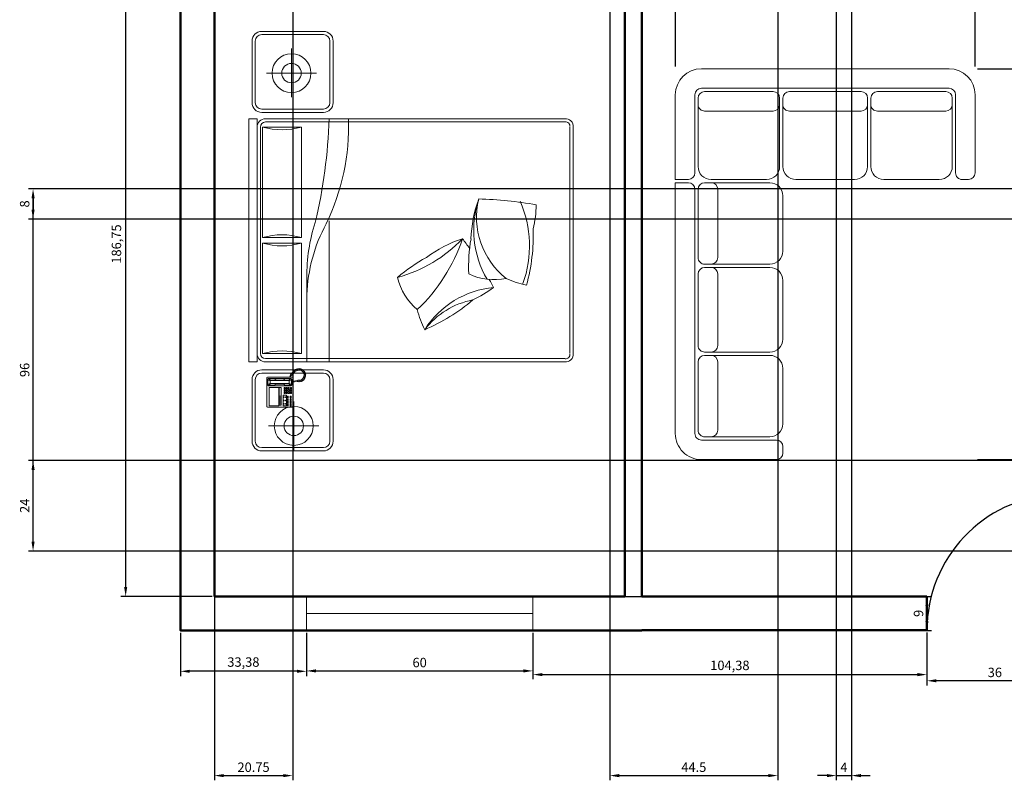
# Model space of a CAD drawing. Units: inches. Extents: x 907 to 2409, y 377 to 1163.
# Tile 1 of 9: x 936 to 1197, y 377 to 579. Entities that reach past the tile are written whole.
import ezdxf

# ---------------------------------------------------------------- set-up
doc = ezdxf.new("R2010")
doc.units = ezdxf.units.IN
for name, color, linetype, lineweight in [('A-ANNO-DIMS', 2, 'Continuous', 18), ('A-DOOR', 3, 'Continuous', 25), ('A-FURN', 8, 'Continuous', 18), ('A-GLAZ', 4, 'Continuous', 18), ('A-WALL', 7, 'Continuous', 50)]:
    doc.layers.add(name, color=color, linetype=linetype, lineweight=lineweight)
doc.styles.get("Standard").update_dxf_attribs({"font": 'arial.ttf'})
doc.dimstyles.new('ISO-25', dxfattribs={"dimtxt": 2.5, "dimasz": 2.5, "dimexe": 1.25, "dimexo": 0.625, "dimtad": 1, "dimtxsty": 'Standard', "dimcen": 2.5, "dimadec": 0, "dimazin": 0, "dimtfac": 1, "dimtmove": 0, "dimatfit": 3, "dimfxl": 1, "dimarcsym": 0})

# ---------------------------------------------------------------- blocks, each defined once
blk = doc.blocks.new('A$C356F0359')
for p, q in [((0.4398, 1.9801), (0.0598, 1.9801)), ((0.4398, 1.9601), (0.0598, 1.9601)), ((0.5489, 2), (2.0492, 2)), ((0.5489, 1.9489), (0.5489, 2)), ((2.0492, 1.9489), (0.5489, 1.9489)), ((2.0492, 1.9489), (2.0492, 2)), ((2.5283, 1.9801), (2.1483, 1.9801)), ((2.5283, 1.9601), (2.1483, 1.9601)), ((-0.0002, 1.9201), (-0.0002, 1.5401)), ((0.0198, 1.9201), (0.0198, 1.5401)), ((0.2725, 1.8879), (0.2702, 1.8856)), ((0.2702, 1.8856), (0.2702, 1.7279)), ((0.2725, 1.8879), (0.4531, 1.8879)), ((0.4016, 1.8787), (0.4062, 1.8845)), ((0.4062, 1.8845), (0.4405, 1.8845)), ((0.4108, 1.8833), (0.4062, 1.881)), ((0.4108, 1.8833), (0.4382, 1.8833)), ((0.4165, 1.8685), (0.4108, 1.8833)), ((0.4325, 1.8685), (0.4382, 1.8833)), ((0.4382, 1.8833), (0.4428, 1.881)), ((0.4405, 1.8845), (0.4462, 1.8787)), ((0.4531, 1.8879), (0.4553, 1.8856)), ((0.4553, 1.8856), (0.4553, 1.7279)), ((0.4798, 1.5401), (0.4798, 1.9201)), ((0.4998, 1.5401), (0.4998, 1.9201)), ((0.5489, 1.8977), (0.5489, 0.0512)), ((0.5689, 1.8977), (0.5689, 0.0512)), ((1.998, 1.9289), (0.6001, 1.9289)), ((2.0292, 0.0512), (2.0292, 1.8977)), ((2.0492, 0.0512), (2.0492, 1.8977)), ((2.0883, 1.9201), (2.0883, 1.5401)), ((2.1083, 1.9201), (2.1083, 1.5401)), ((2.3306, 1.5822), (2.3306, 1.8917)), ((2.5683, 1.5401), (2.5683, 1.9201)), ((2.5883, 1.5401), (2.5883, 1.9201)), ((0.1539, 1.5681), (0.1539, 1.8777)), ((0.3913, 1.8753), (0.277, 1.8753)), ((0.277, 1.8753), (0.277, 1.8147)), ((0.3913, 1.8147), (0.3913, 1.8753)), ((0.4016, 1.7404), (0.4016, 1.8787)), ((0.4062, 1.881), (0.405, 1.8765)), ((0.405, 1.8765), (0.4153, 1.8662)), ((0.405, 1.8765), (0.405, 1.8456)), ((0.405, 1.8456), (0.4073, 1.8399)), ((0.4073, 1.8399), (0.4108, 1.8342)), ((0.4108, 1.8342), (0.4119, 1.8262)), ((0.4119, 1.8262), (0.4119, 1.8147)), ((0.4153, 1.8662), (0.4165, 1.8685)), ((0.4153, 1.8147), (0.4153, 1.8662)), ((0.4325, 1.8685), (0.4165, 1.8685)), ((0.4336, 1.8662), (0.4325, 1.8685)), ((0.4439, 1.8765), (0.4336, 1.8662)), ((0.4336, 1.8147), (0.4336, 1.8662)), ((0.4382, 1.8342), (0.4371, 1.8262)), ((0.4371, 1.8262), (0.4371, 1.8147)), ((0.4416, 1.8399), (0.4382, 1.8342)), ((0.4439, 1.8456), (0.4416, 1.8399)), ((0.4428, 1.881), (0.4439, 1.8765)), ((0.4439, 1.8765), (0.4439, 1.8456)), ((0.4462, 1.8787), (0.4462, 1.7416)), ((0.277, 1.8147), (0.3913, 1.8147)), ((0.277, 1.7885), (0.277, 1.7679)), ((0.3445, 1.7885), (0.277, 1.7885)), ((0.277, 1.7679), (0.3445, 1.7679)), ((0.2782, 1.7622), (0.2782, 1.7576)), ((0.2896, 1.7622), (0.2782, 1.7622)), ((0.3913, 1.8125), (0.2816, 1.8125)), ((0.2816, 1.8125), (0.2816, 1.801)), ((0.2816, 1.801), (0.3913, 1.801)), ((0.2885, 1.7862), (0.2885, 1.7827)), ((0.2919, 1.7862), (0.2885, 1.7862)), ((0.2885, 1.7827), (0.2919, 1.7827)), ((0.2919, 1.7736), (0.2885, 1.7736)), ((0.2885, 1.7736), (0.2885, 1.7702)), ((0.2885, 1.7702), (0.2919, 1.7702)), ((0.2896, 1.7576), (0.2896, 1.7622)), ((0.2907, 1.8125), (0.2907, 1.801)), ((0.2919, 1.7827), (0.2919, 1.7862)), ((0.2919, 1.7702), (0.2919, 1.7736)), ((0.2942, 1.7622), (0.2942, 1.7576)), ((0.3056, 1.7622), (0.2942, 1.7622)), ((0.2999, 1.8125), (0.2999, 1.801)), ((0.3056, 1.7576), (0.3056, 1.7622)), ((0.309, 1.8125), (0.309, 1.801)), ((0.3125, 1.7862), (0.309, 1.7862)), ((0.309, 1.7862), (0.309, 1.7827)), ((0.309, 1.7827), (0.3125, 1.7827)), ((0.3125, 1.7736), (0.309, 1.7736)), ((0.309, 1.7736), (0.309, 1.7702)), ((0.309, 1.7702), (0.3125, 1.7702)), ((0.3102, 1.7622), (0.3102, 1.7576)), ((0.3216, 1.7622), (0.3102, 1.7622)), ((0.3125, 1.7827), (0.3125, 1.7862)), ((0.3125, 1.7702), (0.3125, 1.7736)), ((0.3182, 1.8125), (0.3182, 1.801)), ((0.3216, 1.7576), (0.3216, 1.7622)), ((0.3376, 1.7622), (0.3262, 1.7622)), ((0.3262, 1.7622), (0.3262, 1.7576)), ((0.3273, 1.8125), (0.3273, 1.801)), ((0.333, 1.7862), (0.3296, 1.7862)), ((0.3296, 1.7862), (0.3296, 1.7827)), ((0.3296, 1.7827), (0.333, 1.7827)), ((0.333, 1.7736), (0.3296, 1.7736)), ((0.3296, 1.7736), (0.3296, 1.7702)), ((0.3296, 1.7702), (0.333, 1.7702)), ((0.333, 1.7827), (0.333, 1.7862)), ((0.333, 1.7702), (0.333, 1.7736)), ((0.3365, 1.8125), (0.3365, 1.801)), ((0.3376, 1.7576), (0.3376, 1.7622)), ((0.3445, 1.7679), (0.3445, 1.7885)), ((0.3548, 1.7759), (0.3548, 1.7827)), ((0.3548, 1.7827), (0.3639, 1.7827)), ((0.3639, 1.7759), (0.3548, 1.7759)), ((0.3548, 1.7633), (0.3548, 1.7702)), ((0.3548, 1.7702), (0.3639, 1.7702)), ((0.3639, 1.7633), (0.3548, 1.7633)), ((0.3639, 1.7827), (0.3639, 1.7759)), ((0.3639, 1.7702), (0.3639, 1.7633)), ((0.3685, 1.7827), (0.3776, 1.7827)), ((0.3685, 1.7759), (0.3685, 1.7827)), ((0.3776, 1.7759), (0.3685, 1.7759)), ((0.3685, 1.7633), (0.3685, 1.7702)), ((0.3685, 1.7702), (0.3776, 1.7702)), ((0.3776, 1.7633), (0.3685, 1.7633)), ((0.3776, 1.7827), (0.3776, 1.7759)), ((0.3776, 1.7702), (0.3776, 1.7633)), ((0.3822, 1.7759), (0.3822, 1.7827)), ((0.3822, 1.7827), (0.3913, 1.7827)), ((0.3913, 1.7759), (0.3822, 1.7759)), ((0.3822, 1.7633), (0.3822, 1.7702)), ((0.3822, 1.7702), (0.3913, 1.7702)), ((0.3913, 1.7633), (0.3822, 1.7633)), ((0.3913, 1.801), (0.3913, 1.8125)), ((0.3913, 1.7827), (0.3913, 1.7759)), ((0.3913, 1.7702), (0.3913, 1.7633)), ((0.405, 1.7736), (0.4073, 1.7793)), ((0.405, 1.7427), (0.405, 1.7736)), ((0.4073, 1.7793), (0.4108, 1.785)), ((0.4108, 1.785), (0.4119, 1.793)), ((0.4119, 1.793), (0.4119, 1.8147)), ((0.4153, 1.8147), (0.4153, 1.753)), ((0.4336, 1.8147), (0.4336, 1.753)), ((0.4371, 1.793), (0.4371, 1.8147)), ((0.4382, 1.785), (0.4371, 1.793)), ((0.4416, 1.7793), (0.4382, 1.785)), ((0.4439, 1.7736), (0.4416, 1.7793)), ((0.4439, 1.7427), (0.4439, 1.7736)), ((0.3052, 1.7226), (0.0051, 1.7226)), ((0.2702, 1.7279), (0.2725, 1.7256)), ((0.4244, 1.7256), (0.2725, 1.7256)), ((0.2782, 1.7576), (0.2896, 1.7576)), ((0.2782, 1.745), (0.2896, 1.745)), ((0.2782, 1.7382), (0.2782, 1.745)), ((0.2896, 1.7382), (0.2782, 1.7382)), ((0.2896, 1.745), (0.2896, 1.7382)), ((0.2942, 1.7576), (0.3056, 1.7576)), ((0.2942, 1.745), (0.3056, 1.745)), ((0.2942, 1.7382), (0.2942, 1.745)), ((0.3056, 1.7382), (0.2942, 1.7382)), ((0.3056, 1.745), (0.3056, 1.7382)), ((0.3102, 1.7576), (0.3216, 1.7576)), ((0.3102, 1.745), (0.3216, 1.745)), ((0.3102, 1.7382), (0.3102, 1.745)), ((0.3216, 1.7382), (0.3102, 1.7382)), ((0.3216, 1.745), (0.3216, 1.7382)), ((0.3262, 1.7576), (0.3376, 1.7576)), ((0.3262, 1.7382), (0.3262, 1.745)), ((0.3262, 1.745), (0.3376, 1.745)), ((0.3376, 1.7382), (0.3262, 1.7382)), ((0.3376, 1.745), (0.3376, 1.7382)), ((0.3548, 1.7564), (0.3639, 1.7564)), ((0.3548, 1.7496), (0.3548, 1.7564)), ((0.3639, 1.7496), (0.3548, 1.7496)), ((0.3548, 1.737), (0.3548, 1.7439)), ((0.3548, 1.7439), (0.3639, 1.7439)), ((0.3639, 1.737), (0.3548, 1.737)), ((0.3639, 1.7564), (0.3639, 1.7496)), ((0.3639, 1.7439), (0.3639, 1.737)), ((0.3685, 1.7564), (0.3776, 1.7564)), ((0.3685, 1.7496), (0.3685, 1.7564)), ((0.3776, 1.7496), (0.3685, 1.7496)), ((0.3685, 1.737), (0.3685, 1.7439)), ((0.3685, 1.7439), (0.3776, 1.7439)), ((0.3776, 1.737), (0.3685, 1.737)), ((0.3776, 1.7564), (0.3776, 1.7496)), ((0.3776, 1.7439), (0.3776, 1.737)), ((0.3822, 1.7576), (0.3913, 1.7576)), ((0.3822, 1.7507), (0.3822, 1.7576)), ((0.3913, 1.7507), (0.3822, 1.7507)), ((0.3822, 1.7439), (0.3913, 1.7439)), ((0.3822, 1.737), (0.3822, 1.7439)), ((0.3913, 1.737), (0.3822, 1.737)), ((0.3913, 1.7576), (0.3913, 1.7507)), ((0.3913, 1.7439), (0.3913, 1.737)), ((0.4073, 1.7347), (0.4016, 1.7404)), ((0.405, 1.7427), (0.4153, 1.753)), ((0.4062, 1.7382), (0.405, 1.7427)), ((0.4108, 1.7359), (0.4062, 1.7382)), ((0.4234, 1.7347), (0.4073, 1.7347)), ((0.4165, 1.7507), (0.4108, 1.7359)), ((0.4108, 1.7359), (0.4234, 1.7359)), ((0.4153, 1.753), (0.4165, 1.7507)), ((0.4325, 1.7507), (0.4165, 1.7507)), ((0.4233, 1.7393), (0.4235, 1.7294)), ((0.4268, 1.7393), (0.4233, 1.7393)), ((0.4235, 1.7294), (0.4263, 1.7179)), ((0.4263, 1.7179), (0.429, 1.707)), ((0.4274, 1.7301), (0.4268, 1.7393)), ((0.427, 1.7359), (0.4382, 1.7359)), ((0.4405, 1.7347), (0.4271, 1.7347)), ((0.429, 1.7227), (0.4274, 1.7301)), ((0.4531, 1.7256), (0.4284, 1.7256)), ((0.429, 1.707), (0.4288, 1.701)), ((0.4288, 1.701), (0.4295, 1.6996)), ((0.4318, 1.7119), (0.429, 1.7227)), ((0.4325, 1.7063), (0.4318, 1.7119)), ((0.4323, 1.7003), (0.4325, 1.7063)), ((0.4364, 1.6973), (0.4323, 1.7003)), ((0.4336, 1.753), (0.4325, 1.7507)), ((0.4325, 1.7507), (0.4382, 1.7359)), ((0.4439, 1.7427), (0.4336, 1.753)), ((0.4382, 1.7359), (0.4428, 1.7382)), ((0.4462, 1.7416), (0.4405, 1.7347)), ((0.4428, 1.7382), (0.4439, 1.7427)), ((0.4553, 1.7279), (0.4531, 1.7256)), ((0.4622, 1.7459), (0.4553, 1.7484)), ((0.4553, 1.7439), (0.4604, 1.7425)), ((0.4604, 1.7425), (0.465, 1.7388)), ((0.4654, 1.7427), (0.4622, 1.7459)), ((0.465, 1.7388), (0.4662, 1.7372)), ((0.4678, 1.7405), (0.4654, 1.7427)), ((0.4662, 1.7372), (0.4686, 1.7374)), ((0.4686, 1.7374), (0.4662, 1.735)), ((0.4662, 1.735), (0.4755, 1.7268)), ((0.4721, 1.7421), (0.4678, 1.7405)), ((0.4741, 1.7401), (0.4721, 1.7421)), ((0.4725, 1.7366), (0.4741, 1.7401)), ((0.4753, 1.7388), (0.4725, 1.7366)), ((0.4783, 1.7356), (0.4753, 1.7388)), ((0.4755, 1.7268), (0.4906, 1.7139)), ((0.4759, 1.729), (0.4783, 1.7356)), ((0.4821, 1.7322), (0.4759, 1.729)), ((0.4874, 1.7272), (0.4821, 1.7322)), ((0.4862, 1.7199), (0.4874, 1.7272)), ((0.4914, 1.7231), (0.4862, 1.7199)), ((0.4908, 1.7135), (0.4984, 1.6917)), ((0.4958, 1.7185), (0.4914, 1.7231)), ((0.494, 1.7135), (0.4958, 1.7185)), ((0.501, 1.7142), (0.494, 1.7135)), ((0.4964, 1.7047), (0.5031, 1.7072)), ((0.5038, 1.7049), (0.4964, 1.7047)), ((0.5031, 1.7072), (0.501, 1.7142)), ((0.5054, 1.6996), (0.5038, 1.7049)), ((2.4819, 1.7366), (2.1818, 1.7366)), ((0.427, 1.697), (0.4265, 1.6915)), ((0.4265, 1.6915), (0.4332, 1.6903)), ((0.4332, 1.6903), (0.4267, 1.6864)), ((0.4267, 1.6864), (0.4272, 1.6801)), ((0.4295, 1.6996), (0.427, 1.697)), ((0.4272, 1.6801), (0.4346, 1.6794)), ((0.4346, 1.6794), (0.4281, 1.6744)), ((0.4281, 1.6744), (0.4311, 1.669)), ((0.4311, 1.669), (0.4381, 1.6704)), ((0.4381, 1.6704), (0.4348, 1.6639)), ((0.4348, 1.6639), (0.4383, 1.6598)), ((0.4355, 1.6919), (0.4364, 1.6973)), ((0.4367, 1.6774), (0.4355, 1.6919)), ((0.4455, 1.6663), (0.4367, 1.6774)), ((0.4383, 1.6598), (0.4436, 1.6637)), ((0.4436, 1.6637), (0.4427, 1.6575)), ((0.4427, 1.6575), (0.4471, 1.6547)), ((0.4577, 1.6598), (0.4455, 1.6663)), ((0.4471, 1.6547), (0.4526, 1.6593)), ((0.4526, 1.6593), (0.4519, 1.6517)), ((0.4519, 1.6517), (0.4568, 1.6503)), ((0.4568, 1.6503), (0.4598, 1.6565)), ((0.4716, 1.6586), (0.4577, 1.6598)), ((0.4598, 1.6565), (0.4626, 1.6503)), ((0.4626, 1.6503), (0.4665, 1.6498)), ((0.4665, 1.6498), (0.4681, 1.6565)), ((0.4681, 1.6565), (0.4707, 1.6491)), ((0.4707, 1.6491), (0.4751, 1.6503)), ((0.485, 1.6644), (0.4716, 1.6586)), ((0.4751, 1.6503), (0.4753, 1.6565)), ((0.4753, 1.6565), (0.4806, 1.6519)), ((0.4806, 1.6519), (0.4843, 1.6538)), ((0.4843, 1.6538), (0.4836, 1.6607)), ((0.4836, 1.6607), (0.4885, 1.6547)), ((0.4952, 1.6744), (0.485, 1.6644)), ((0.4885, 1.6547), (0.4922, 1.6579)), ((0.4922, 1.6579), (0.4894, 1.6642)), ((0.4894, 1.6642), (0.4959, 1.6614)), ((0.4984, 1.6917), (0.4952, 1.6744)), ((0.4957, 1.6704), (0.5024, 1.6683)), ((0.4989, 1.6642), (0.4957, 1.6704)), ((0.4959, 1.6614), (0.4989, 1.6642)), ((0.5042, 1.673), (0.4987, 1.6792)), ((0.4987, 1.6792), (0.5058, 1.679)), ((0.5005, 1.695), (0.5054, 1.6996)), ((0.5068, 1.695), (0.5005, 1.695)), ((0.5008, 1.6871), (0.5079, 1.6892)), ((0.5068, 1.6836), (0.5008, 1.6871)), ((0.5024, 1.6683), (0.5042, 1.673)), ((0.5058, 1.679), (0.5068, 1.6836)), ((0.5079, 1.6892), (0.5068, 1.695)), ((0.0598, 1.5001), (0.4398, 1.5001)), ((0.0598, 1.4801), (0.4398, 1.4801)), ((2.1483, 1.5001), (2.5283, 1.5001)), ((2.1483, 1.4801), (2.5283, 1.4801)), ((0.6001, 0.02), (1.998, 0.02)), ((0.6001, 0), (1.998, 0))]:
    blk.add_line(p, q)
at = {"linetype": 'ByBlock'}
for p, q in [((0.6001, 1.9147), (1.282, 1.9147)), ((0.6001, 1.6759), (0.6001, 1.9147)), ((1.282, 1.9147), (1.282, 1.6759)), ((1.3161, 1.9147), (1.998, 1.9147)), ((1.3161, 1.6759), (1.3161, 1.9147)), ((1.998, 1.9147), (1.998, 1.6759)), ((1.0687, 1.6418), (0.5489, 1.6418)), ((1.282, 1.6759), (0.6001, 1.6759)), ((1.998, 1.6759), (1.3161, 1.6759)), ((1.4185, 1.5053), (0.5489, 1.5053))]:
    blk.add_line(p, q, dxfattribs=at)
for centre in [(0.1539, 1.7226), (2.3306, 1.7366)]:
    blk.add_circle(centre, 0.12, dxfattribs=at)
for centre in [(0.1539, 1.7226), (2.3306, 1.7366)]:
    blk.add_circle(centre, 0.06)
for centre, radius, start, end in [((0.0598, 1.9201), 0.06, 90, 180), ((0.0598, 1.9201), 0.04, 90, 180), ((0.4398, 1.9201), 0.06, 0, 90), ((0.4398, 1.9201), 0.04, 0, 90), ((0.6001, 1.8977), 0.0512, 90, 180), ((1.998, 1.8977), 0.0512, 0, 90), ((2.1483, 1.9201), 0.06, 90, 180), ((2.1483, 1.9201), 0.04, 90, 180), ((2.5283, 1.9201), 0.06, 0, 90), ((2.5283, 1.9201), 0.04, 0, 90), ((0.6001, 1.8977), 0.0312, 90, 180), ((1.998, 1.8977), 0.0312, 0, 90), ((0.0598, 1.5401), 0.06, 180, 270), ((0.0598, 1.5401), 0.04, 180, 270), ((0.4398, 1.5401), 0.04, 270, 0), ((0.4398, 1.5401), 0.06, 270, 0), ((2.1483, 1.5401), 0.06, 180, 270), ((2.1483, 1.5401), 0.04, 180, 270), ((2.5283, 1.5401), 0.06, 270, 0), ((2.5283, 1.5401), 0.04, 270, 0), ((1.1471, 0.7332), 0.3575, 102.47819, 140.46254), ((1.9086, 1.3124), 0.8697, 195.33601, 226.41927), ((0.3249, 0.4335), 0.9879, 28.49711, 41.05657), ((0.9965, 0.4273), 0.548, 103.20343, 117.03623), ((0.4451, 0.4375), 0.5655, 5.33912, 57.68949), ((0.4517, 0.5274), 0.4879, 10.69865, 52.68638), ((1.8195, 1.3719), 1.1652, 203.06416, 220.32086), ((1.6529, 1.7059), 1.0798, 223.63057, 251.4288), ((0.5617, 0.4344), 0.7874, 18.35266, 36.68512), ((-0.021, 2.4319), 2.1977, 305.29657, 307.24182), ((1.5949, 0.9312), 0.734, 205.25901, 216.93514), ((1.4135, 0.487), 0.3575, 154.0418, 192.02615), ((1.3641, 0.0041), 0.6085, 71.81005, 120.13512), ((1.1372, -0.3434), 0.9879, 80.06073, 92.62018), ((1.2836, -0.1573), 0.7874, 69.91627, 88.24873), ((1.44, 0.1186), 0.4774, 76.18494, 142.00166), ((-0.6432, 0.628), 2.1977, 349.48843, 358.80544), ((-0.021, 2.4319), 2.1977, 297.92482, 299.3793), ((1.5595, 0.1789), 0.548, 154.76704, 168.59984), ((1.2647, 0.9578), 0.6885, 250.29361, 293.6414), ((1.3312, 1.4107), 1.1652, 254.62778, 271.88448), ((1.5368, 0.9609), 0.734, 256.82263, 268.49876), ((0.5943, 0.0454), 0.0458, 172.75992, 277.24008), ((0.5943, 0.0454), 0.0258, 172.75992, 277.24008), ((2.0038, 0.0454), 0.0458, 262.75992, 7.24008), ((2.0038, 0.0454), 0.0258, 262.75992, 7.24008)]:
    blk.add_arc(centre, radius, start, end)
for centre, radius, start, end in [((0.1906, 1.7953), 0.4265, 343.73979, 16.26021), ((1.6914, 1.7953), 0.4265, 163.73979, 196.26021), ((0.9067, 1.7953), 0.4265, 343.73979, 16.26021), ((2.4075, 1.7953), 0.4265, 163.73979, 196.26021), ((0.9303, 0.657), 0.9853, 61.43285, 88.12613), ((1.0826, 0.5712), 1.0706, 72.19663, 90.74184), ((2.1368, 4.5996), 3.0955, 256.42012, 268.37887), ((2.0056, 2.7745), 1.3903, 244.24266, 271.79845)]:
    blk.add_arc(centre, radius, start, end, dxfattribs=at)
blk = doc.blocks.new('A$C2AFA021D')
for p, q in [((0.8, 2.3), (0.2, 2.3)), ((0.85, 2.2), (0.85, 2.25)), ((0.2, 2.15), (0.8, 2.15)), ((0.225, 2.125), (0.275, 2.125)), ((0.75, 2.125), (0.275, 2.125)), ((0, 2.1), (0, 0.2)), ((0.15, 0.2), (0.15, 2.1)), ((0.175, 1.55), (0.175, 2.075)), ((0.325, 2.075), (0.325, 1.55)), ((0.85, 1.6), (0.85, 2.025)), ((0.275, 1.5), (0.225, 1.5)), ((0.225, 1.475), (0.275, 1.475)), ((0.275, 1.5), (0.75, 1.5)), ((0.75, 1.475), (0.275, 1.475)), ((0.175, 0.875), (0.175, 1.425)), ((0.325, 1.425), (0.325, 0.875)), ((0.85, 0.925), (0.85, 1.375)), ((0.275, 0.825), (0.225, 0.825)), ((0.225, 0.8), (0.275, 0.8)), ((0.275, 0.825), (0.75, 0.825)), ((0.75, 0.8), (0.275, 0.8)), ((0.975, 0.825), (1.4, 0.825)), ((1.625, 0.825), (2.075, 0.825)), ((2.3, 0.825), (2.725, 0.825)), ((2.85, 0.2), (2.85, 0.775)), ((2.9, 0.825), (2.95, 0.825)), ((3, 0.775), (3, 0.2)), ((0.175, 0.225), (0.175, 0.75)), ((0.325, 0.75), (0.325, 0.225)), ((0.85, 0.275), (0.85, 0.7)), ((0.875, 0.275), (0.875, 0.725)), ((1.5, 0.725), (1.5, 0.275)), ((1.525, 0.275), (1.525, 0.725)), ((2.175, 0.725), (2.175, 0.275)), ((2.2, 0.275), (2.2, 0.725)), ((2.825, 0.725), (2.825, 0.275)), ((1.45, 0.325), (0.925, 0.325)), ((2.125, 0.325), (1.575, 0.325)), ((2.775, 0.325), (2.25, 0.325)), ((0.875, 0.275), (0.875, 0.225)), ((1.5, 0.225), (1.5, 0.275)), ((1.525, 0.275), (1.525, 0.225)), ((2.175, 0.225), (2.175, 0.275)), ((2.2, 0.275), (2.2, 0.225)), ((2.825, 0.225), (2.825, 0.275)), ((0.275, 0.175), (0.225, 0.175)), ((0.275, 0.175), (0.75, 0.175)), ((0.925, 0.175), (1.45, 0.175)), ((1.575, 0.175), (2.125, 0.175)), ((2.25, 0.175), (2.775, 0.175)), ((0.8, 0.15), (0.2, 0.15)), ((0.85, 0), (0.85, 0.1)), ((0.875, 0.1), (0.875, 0)), ((0.925, 0.15), (2.8, 0.15)), ((0.2, 0), (0.85, 0)), ((2.8, 0), (0.875, 0))]:
    blk.add_line(p, q)
for centre, radius, start, end in [((0.2, 2.1), 0.2, 90, 180), ((0.8, 2.25), 0.05, 0, 90), ((0.8, 2.2), 0.05, 270, 0), ((0.2, 2.1), 0.05, 90, 180), ((0.225, 2.075), 0.05, 90, 180), ((0.275, 2.075), 0.05, 0, 90), ((0.75, 2.025), 0.1, 0, 90), ((0.75, 1.6), 0.1, 270, 0), ((0.225, 1.55), 0.05, 180, 270), ((0.275, 1.55), 0.05, 270, 0), ((0.225, 1.425), 0.05, 90, 180), ((0.275, 1.425), 0.05, 0, 90), ((0.75, 1.375), 0.1, 360, 90), ((0.75, 0.925), 0.1, 270, 0), ((0.225, 0.875), 0.05, 180, 270), ((0.275, 0.875), 0.05, 270, 0), ((0.225, 0.75), 0.05, 90, 180), ((0.275, 0.75), 0.05, 0, 90), ((0.75, 0.7), 0.1, 0, 90), ((0.975, 0.725), 0.1, 90, 180), ((1.4, 0.725), 0.1, 0, 90), ((1.625, 0.725), 0.1, 90, 180), ((2.075, 0.725), 0.1, 0, 90), ((2.3, 0.725), 0.1, 90, 180), ((2.725, 0.725), 0.1, 0, 90), ((2.9, 0.775), 0.05, 90, 180), ((2.95, 0.775), 0.05, 0, 90), ((0.925, 0.275), 0.05, 90, 180), ((1.45, 0.275), 0.05, 360, 90), ((1.575, 0.275), 0.05, 90, 180), ((2.125, 0.275), 0.05, 360, 90), ((2.25, 0.275), 0.05, 90, 180), ((2.775, 0.275), 0.05, 360, 90), ((0.75, 0.275), 0.1, 270, 0), ((0.2, 0.2), 0.2, 180, 270), ((0.2, 0.2), 0.05, 180, 270), ((0.225, 0.225), 0.05, 180, 270), ((0.275, 0.225), 0.05, 270, 0), ((0.925, 0.225), 0.05, 180, 270), ((1.45, 0.225), 0.05, 270, 0), ((1.575, 0.225), 0.05, 180, 270), ((2.125, 0.225), 0.05, 270, 0), ((2.25, 0.225), 0.05, 180, 270), ((2.775, 0.225), 0.05, 270, 0), ((2.8, 0.2), 0.2, 270, 0), ((2.8, 0.2), 0.05, 270, 0), ((0.8, 0.1), 0.05, 0, 90), ((0.925, 0.1), 0.05, 90, 180)]:
    blk.add_arc(centre, radius, start, end)
blk = doc.blocks.new('*D24')
at = {"layer": 'A-ANNO-DIMS', "color": 0, "lineweight": -2, "transparency": 16777216}
for p, q in [((1176.36, 416.32), (1176.36, 402.25)), ((1212.36, 416.25), (1212.36, 402.25)), ((1209.86, 403.5), (1178.86, 403.5))]:
    blk.add_line(p, q, dxfattribs=at)
at = {"layer": 'A-ANNO-DIMS', "color": 0, "transparency": 16777216}
for points in [[(1178.86, 403.92), (1178.86, 403.09), (1176.36, 403.5)], [(1209.86, 403.92), (1209.86, 403.09), (1212.36, 403.5)]]:
    blk.add_solid(points, dxfattribs=at)
at = {"layer": 'Defpoints', "color": 0, "transparency": 16777216}
for p in [(1176.36, 416.95), (1212.36, 416.87), (1176.36, 403.5)]:
    blk.add_point(p, dxfattribs=at)
at = {"layer": 'A-ANNO-DIMS', "color": 0, "transparency": 16777216, "insert": (1194.36, 405.4), "char_height": 2.5, "attachment_point": 5}
blk.add_mtext('36', dxfattribs=at)
blk = doc.blocks.new('*D25')
at = {"layer": 'A-ANNO-DIMS', "color": 0, "lineweight": -2, "transparency": 16777216}
for p, q in [((1072.61, 425.87), (1177.61, 425.87)), ((1176.36, 423.37), (1176.36, 419.37)), ((1072.61, 416.87), (1177.61, 416.87))]:
    blk.add_line(p, q, dxfattribs=at)
at = {"layer": 'A-ANNO-DIMS', "color": 0, "transparency": 16777216}
for points in [[(1175.95, 423.37), (1176.78, 423.37), (1176.36, 425.87)], [(1175.95, 419.37), (1176.78, 419.37), (1176.36, 416.87)]]:
    blk.add_solid(points, dxfattribs=at)
at = {"layer": 'Defpoints', "color": 0, "transparency": 16777216}
for p in [(1071.99, 425.87), (1071.99, 416.87), (1176.36, 416.87)]:
    blk.add_point(p, dxfattribs=at)
at = {"layer": 'A-ANNO-DIMS', "color": 0, "transparency": 16777216, "insert": (1174.46, 421.37), "char_height": 2.5, "attachment_point": 5, "rotation": 90}
blk.add_mtext('9', dxfattribs=at)
blk = doc.blocks.new('*D26')
at = {"layer": 'A-ANNO-DIMS', "color": 0, "lineweight": -2, "transparency": 16777216}
for p, q in [((1071.99, 416.25), (1071.99, 403.89)), ((1176.36, 416.25), (1176.36, 403.89)), ((1074.49, 405.14), (1173.86, 405.14))]:
    blk.add_line(p, q, dxfattribs=at)
at = {"layer": 'A-ANNO-DIMS', "color": 0, "transparency": 16777216}
for points in [[(1074.49, 405.55), (1074.49, 404.72), (1071.99, 405.14)], [(1173.86, 405.55), (1173.86, 404.72), (1176.36, 405.14)]]:
    blk.add_solid(points, dxfattribs=at)
at = {"layer": 'Defpoints', "color": 0, "transparency": 16777216}
for p in [(1071.99, 416.87), (1176.36, 416.87), (1176.36, 405.14)]:
    blk.add_point(p, dxfattribs=at)
at = {"layer": 'A-ANNO-DIMS', "color": 0, "transparency": 16777216, "insert": (1124.17, 407.26), "char_height": 2.5, "attachment_point": 5}
blk.add_mtext('104,38', dxfattribs=at)
blk = doc.blocks.new('*D27')
at = {"layer": 'A-ANNO-DIMS', "color": 0, "lineweight": -2, "transparency": 16777216}
for p, q in [((1011.99, 416.25), (1011.99, 404.86)), ((1071.99, 416.25), (1071.99, 404.86)), ((1014.49, 406.11), (1069.49, 406.11))]:
    blk.add_line(p, q, dxfattribs=at)
at = {"layer": 'A-ANNO-DIMS', "color": 0, "transparency": 16777216}
for points in [[(1014.49, 406.53), (1014.49, 405.7), (1011.99, 406.11)], [(1069.49, 406.53), (1069.49, 405.7), (1071.99, 406.11)]]:
    blk.add_solid(points, dxfattribs=at)
at = {"layer": 'Defpoints', "color": 0, "transparency": 16777216}
for p in [(1011.99, 416.87), (1071.99, 416.87), (1071.99, 406.11)]:
    blk.add_point(p, dxfattribs=at)
at = {"layer": 'A-ANNO-DIMS', "color": 0, "transparency": 16777216, "insert": (1041.99, 408.01), "char_height": 2.5, "attachment_point": 5}
blk.add_mtext('60', dxfattribs=at)
blk = doc.blocks.new('*D28')
at = {"layer": 'A-ANNO-DIMS', "color": 0, "lineweight": -2, "transparency": 16777216}
for p, q in [((978.61, 416.25), (978.61, 404.76)), ((1011.99, 416.25), (1011.99, 404.76)), ((1009.49, 406.01), (981.11, 406.01))]:
    blk.add_line(p, q, dxfattribs=at)
at = {"layer": 'A-ANNO-DIMS', "color": 0, "transparency": 16777216}
for points in [[(981.11, 406.43), (981.11, 405.6), (978.61, 406.01)], [(1009.49, 406.43), (1009.49, 405.6), (1011.99, 406.01)]]:
    blk.add_solid(points, dxfattribs=at)
at = {"layer": 'Defpoints', "color": 0, "transparency": 16777216}
for p in [(978.61, 416.87), (1011.99, 416.87), (978.61, 406.01)]:
    blk.add_point(p, dxfattribs=at)
at = {"layer": 'A-ANNO-DIMS', "color": 0, "transparency": 16777216, "insert": (995.3, 408.14), "char_height": 2.5, "attachment_point": 5}
blk.add_mtext('33,38', dxfattribs=at)
blk = doc.blocks.new('*D37')
at = {"layer": 'A-ANNO-DIMS', "color": 0, "lineweight": -2, "transparency": 16777216}
for p, q in [((986.99, 612.62), (962.87, 612.62)), ((964.12, 428.37), (964.12, 610.12)), ((986.99, 425.87), (962.87, 425.87))]:
    blk.add_line(p, q, dxfattribs=at)
at = {"layer": 'A-ANNO-DIMS', "color": 0, "transparency": 16777216}
for points in [[(963.7, 610.12), (964.53, 610.12), (964.12, 612.62)], [(963.7, 428.37), (964.53, 428.37), (964.12, 425.87)]]:
    blk.add_solid(points, dxfattribs=at)
at = {"layer": 'Defpoints', "color": 0, "transparency": 16777216}
for p in [(964.12, 612.62), (987.61, 612.62), (987.61, 425.87)]:
    blk.add_point(p, dxfattribs=at)
at = {"layer": 'A-ANNO-DIMS', "color": 0, "transparency": 16777216, "insert": (961.99, 519.25), "char_height": 2.5, "attachment_point": 5, "rotation": 90}
blk.add_mtext('186,75', dxfattribs=at)
blk = doc.blocks.new('DOOR-36IN')
for p, q in [((36, 36), (36, 0)), ((36, 0), (34, 0)), ((36, 0), (34, 0))]:
    blk.add_line(p, q)
blk.add_lwpolyline([(36, 36), (34, 36), (34, 0), (36, 0)], close=True)
blk.add_arc((36.06, 0), 36.06, 93.2732, 180)
blk = doc.blocks.new('WIN-60IN')
for p, q in [((0, 9), (0, 0)), ((0, 4.5), (60, 4.5)), ((0, 0), (60, 0))]:
    blk.add_line(p, q)
blk.add_lwpolyline([(0, 9), (60, 9), (60, 0), (0, 0)], close=True)
blk = doc.blocks.new('*D55')
at = {"layer": 'A-ANNO-DIMS', "color": 0, "lineweight": -2, "transparency": 16777216}
for p, q in [((1189.76, 565.7), (1205.92, 565.7)), ((1204.67, 563.2), (1204.67, 464.62)), ((1189.76, 462.12), (1205.92, 462.12))]:
    blk.add_line(p, q, dxfattribs=at)
at = {"layer": 'A-ANNO-DIMS', "color": 0, "transparency": 16777216}
for points in [[(1204.25, 563.2), (1205.09, 563.2), (1204.67, 565.7)], [(1204.25, 464.62), (1205.09, 464.62), (1204.67, 462.12)]]:
    blk.add_solid(points, dxfattribs=at)
at = {"layer": 'Defpoints', "color": 0, "transparency": 16777216}
for p in [(1189.13, 565.7), (1189.13, 462.12), (1204.67, 462.12)]:
    blk.add_point(p, dxfattribs=at)
at = {"layer": 'A-ANNO-DIMS', "color": 0, "transparency": 16777216, "insert": (1202.75, 513.91), "char_height": 2.5, "attachment_point": 5, "rotation": 90}
blk.add_mtext('SOFA 104', dxfattribs=at)
blk = doc.blocks.new('*D56')
at = {"layer": 'A-ANNO-DIMS', "color": 0, "lineweight": -2, "transparency": 16777216}
for p, q in [((1109.72, 566.33), (1109.72, 582.49)), ((1189.13, 566.33), (1189.13, 582.49)), ((1112.22, 581.24), (1186.63, 581.24))]:
    blk.add_line(p, q, dxfattribs=at)
at = {"layer": 'A-ANNO-DIMS', "color": 0, "transparency": 16777216}
for points in [[(1112.22, 581.66), (1112.22, 580.83), (1109.72, 581.24)], [(1186.63, 581.66), (1186.63, 580.83), (1189.13, 581.24)]]:
    blk.add_solid(points, dxfattribs=at)
at = {"layer": 'Defpoints', "color": 0, "transparency": 16777216}
for p in [(1189.13, 581.24), (1109.72, 565.7), (1189.13, 565.7)]:
    blk.add_point(p, dxfattribs=at)
at = {"layer": 'A-ANNO-DIMS', "color": 0, "transparency": 16777216, "insert": (1149.42, 583.14), "char_height": 2.5, "attachment_point": 5}
blk.add_mtext('79', dxfattribs=at)
blk = doc.blocks.new('*D62')
at = {"layer": 'A-ANNO-DIMS', "color": 0, "lineweight": -2, "transparency": 16777216}
for p, q in [((987.61, 426.5), (987.61, 1056.62)), ((1096.36, 426.5), (1096.36, 1056.62)), ((990.11, 1055.37), (1093.86, 1055.37))]:
    blk.add_line(p, q, dxfattribs=at)
at = {"layer": 'A-ANNO-DIMS', "color": 0, "transparency": 16777216}
for points in [[(990.11, 1055.79), (990.11, 1054.95), (987.61, 1055.37)], [(1093.86, 1055.79), (1093.86, 1054.95), (1096.36, 1055.37)]]:
    blk.add_solid(points, dxfattribs=at)
at = {"layer": 'Defpoints', "color": 0, "transparency": 16777216}
for p in [(1096.36, 1055.37), (987.61, 425.87), (1096.36, 425.87)]:
    blk.add_point(p, dxfattribs=at)
at = {"layer": 'A-ANNO-DIMS', "color": 0, "transparency": 16777216, "insert": (1041.99, 1057.27), "char_height": 2.5, "attachment_point": 5}
blk.add_mtext('108.75', dxfattribs=at)
blk = doc.blocks.new('*D64')
at = {"layer": 'A-ANNO-DIMS', "color": 0, "lineweight": -2, "transparency": 16777216}
for p, q in [((1269.47, 533.88), (938.33, 533.88)), ((939.58, 440.38), (939.58, 531.38)), ((1269.47, 437.88), (938.33, 437.88))]:
    blk.add_line(p, q, dxfattribs=at)
at = {"layer": 'A-ANNO-DIMS', "color": 0, "transparency": 16777216}
for points in [[(939.17, 531.38), (940, 531.38), (939.58, 533.88)], [(939.17, 440.38), (940, 440.38), (939.58, 437.88)]]:
    blk.add_solid(points, dxfattribs=at)
at = {"layer": 'Defpoints', "color": 0, "transparency": 16777216}
for p in [(939.58, 533.88), (1270.1, 533.88), (1270.1, 437.88)]:
    blk.add_point(p, dxfattribs=at)
at = {"layer": 'A-ANNO-DIMS', "color": 0, "transparency": 16777216, "insert": (937.68, 485.88), "char_height": 2.5, "attachment_point": 5, "rotation": 90}
blk.add_mtext('96', dxfattribs=at)
blk = doc.blocks.new('*D76')
at = {"layer": 'A-ANNO-DIMS', "color": 0, "lineweight": -2, "transparency": 16777216}
for p, q in [((1269.47, 533.88), (938.33, 533.88)), ((939.58, 531.38), (939.58, 528.38)), ((1269.47, 525.88), (938.33, 525.88))]:
    blk.add_line(p, q, dxfattribs=at)
at = {"layer": 'A-ANNO-DIMS', "color": 0, "transparency": 16777216}
for points in [[(939.17, 531.38), (940, 531.38), (939.58, 533.88)], [(939.17, 528.38), (940, 528.38), (939.58, 525.88)]]:
    blk.add_solid(points, dxfattribs=at)
at = {"layer": 'Defpoints', "color": 0, "transparency": 16777216}
for p in [(1270.1, 533.88), (939.58, 525.88), (1270.1, 525.88)]:
    blk.add_point(p, dxfattribs=at)
at = {"layer": 'A-ANNO-DIMS', "color": 0, "transparency": 16777216, "insert": (937.68, 529.88), "char_height": 2.5, "attachment_point": 5, "rotation": 90}
blk.add_mtext('8', dxfattribs=at)
blk = doc.blocks.new('*D79')
at = {"layer": 'A-ANNO-DIMS', "color": 0, "lineweight": -2, "transparency": 16777216}
for p, q in [((1269.47, 461.88), (938.33, 461.88)), ((939.58, 440.38), (939.58, 459.38)), ((1269.47, 437.88), (938.33, 437.88))]:
    blk.add_line(p, q, dxfattribs=at)
at = {"layer": 'A-ANNO-DIMS', "color": 0, "transparency": 16777216}
for points in [[(939.17, 459.38), (940, 459.38), (939.58, 461.88)], [(939.17, 440.38), (940, 440.38), (939.58, 437.88)]]:
    blk.add_solid(points, dxfattribs=at)
at = {"layer": 'Defpoints', "color": 0, "transparency": 16777216}
for p in [(939.58, 461.88), (1270.1, 461.88), (1270.1, 437.88)]:
    blk.add_point(p, dxfattribs=at)
at = {"layer": 'A-ANNO-DIMS', "color": 0, "transparency": 16777216, "insert": (937.7, 449.88), "char_height": 2.5, "attachment_point": 5, "rotation": 90}
blk.add_mtext('24', dxfattribs=at)
blk = doc.blocks.new('*D82')
at = {"layer": 'A-ANNO-DIMS', "color": 0, "lineweight": -2, "transparency": 16777216}
for p, q in [((987.61, 616.5), (987.61, 377.12)), ((1008.36, 616.5), (1008.36, 377.12)), ((990.11, 378.37), (1005.86, 378.37))]:
    blk.add_line(p, q, dxfattribs=at)
at = {"layer": 'A-ANNO-DIMS', "color": 0, "transparency": 16777216}
for points in [[(990.11, 378.79), (990.11, 377.95), (987.61, 378.37)], [(1005.86, 378.79), (1005.86, 377.95), (1008.36, 378.37)]]:
    blk.add_solid(points, dxfattribs=at)
at = {"layer": 'Defpoints', "color": 0, "transparency": 16777216}
for p in [(987.61, 617.12), (1008.36, 617.12), (1008.36, 378.37)]:
    blk.add_point(p, dxfattribs=at)
at = {"layer": 'A-ANNO-DIMS', "color": 0, "transparency": 16777216, "insert": (997.99, 380.27), "char_height": 2.5, "attachment_point": 5}
blk.add_mtext('20.75', dxfattribs=at)
blk = doc.blocks.new('*D83')
at = {"layer": 'A-ANNO-DIMS', "color": 0, "lineweight": -2, "transparency": 16777216}
for p, q in [((1092.36, 616.5), (1092.36, 377.12)), ((1136.86, 616.5), (1136.86, 377.12)), ((1094.86, 378.37), (1134.36, 378.37))]:
    blk.add_line(p, q, dxfattribs=at)
at = {"layer": 'A-ANNO-DIMS', "color": 0, "transparency": 16777216}
for points in [[(1094.86, 378.79), (1094.86, 377.95), (1092.36, 378.37)], [(1134.36, 378.79), (1134.36, 377.95), (1136.86, 378.37)]]:
    blk.add_solid(points, dxfattribs=at)
at = {"layer": 'Defpoints', "color": 0, "transparency": 16777216}
for p in [(1092.36, 617.12), (1136.86, 617.12), (1136.86, 378.37)]:
    blk.add_point(p, dxfattribs=at)
at = {"layer": 'A-ANNO-DIMS', "color": 0, "transparency": 16777216, "insert": (1114.61, 380.27), "char_height": 2.5, "attachment_point": 5}
blk.add_mtext('44.5', dxfattribs=at)
blk = doc.blocks.new('*D84')
at = {"layer": 'A-ANNO-DIMS', "color": 0, "lineweight": -2, "transparency": 16777216}
for p, q in [((1152.36, 772.5), (1152.36, 377.12)), ((1156.36, 772.5), (1156.36, 377.12)), ((1149.86, 378.37), (1147.36, 378.37)), ((1152.36, 378.37), (1156.36, 378.37)), ((1158.86, 378.37), (1161.36, 378.37))]:
    blk.add_line(p, q, dxfattribs=at)
at = {"layer": 'A-ANNO-DIMS', "color": 0, "transparency": 16777216}
for points in [[(1149.86, 378.79), (1149.86, 377.95), (1152.36, 378.37)], [(1158.86, 378.79), (1158.86, 377.95), (1156.36, 378.37)]]:
    blk.add_solid(points, dxfattribs=at)
at = {"layer": 'Defpoints', "color": 0, "transparency": 16777216}
for p in [(1152.36, 773.12), (1156.36, 773.12), (1156.36, 378.37)]:
    blk.add_point(p, dxfattribs=at)
at = {"layer": 'A-ANNO-DIMS', "color": 0, "transparency": 16777216, "insert": (1154.36, 380.25), "char_height": 2.5, "attachment_point": 5}
blk.add_mtext('4', dxfattribs=at)

msp = doc.modelspace()

# ---------------------------------------------------------------- linework, layer by layer
at = {"layer": 'A-WALL'}
for p, q in [((978.6122, 1016.8705), (978.6122, 416.8705)), ((978.6122, 614.8705), (978.6122, 416.8705)), ((987.6122, 612.6205), (987.6122, 425.8705)), ((1096.3622, 612.6205), (1096.3622, 425.8705)), ((1100.8622, 612.6205), (1100.8622, 425.8705)), ((1011.9872, 425.8705), (987.6122, 425.8705)), ((987.6122, 425.8705), (1096.3622, 425.8705)), ((1100.8622, 425.8705), (1173.1859, 425.8705)), ((1140.6124, 425.945), (1140.6124, 425.8705)), ((1176.3622, 425.8705), (1173.1859, 425.8705)), ((1176.3622, 416.8705), (1176.3622, 425.8705)), ((978.6122, 416.8705), (1100.8622, 416.8705)), ((978.6122, 416.8705), (1100.8622, 416.8705)), ((987.6122, 416.8705), (1096.3622, 416.8705)), ((1140.6124, 416.945), (1100.8622, 416.945)), ((1100.8622, 416.945), (1100.8622, 416.8705))]:
    msp.add_line(p, q, dxfattribs=at)
msp.add_lwpolyline([(1216.3622, 416.8705), (1338.6122, 416.8705), (1338.6122, 1016.8705), (978.6122, 1016.8705), (978.6122, 416.8705), (1100.8622, 416.8705)], dxfattribs=at)
msp.add_lwpolyline([(1140.6124, 416.945), (1176.3622, 416.945), (1176.3622, 416.9079), (1140.6124, 416.9079)], close=True, dxfattribs=at)

# ---------------------------------------------------------------- block references
at = {"layer": 'A-DOOR'}
msp.add_blockref('DOOR-36IN', (1176.3622, 416.8705), dxfattribs=at)
at = {"layer": 'A-FURN'}
for name, p, xscale, yscale, zscale, rotation in [('A$C356F0359', (1082.6383, 464.4384), 42.95257138859579, 42.95257138859579, 42.95257138859579, 90), ('A$C2AFA021D', (1109.7159, 565.7049), 34.52830128526068, 34.52830128526068, 34.52830128526068, 270)]:
    msp.add_blockref(name, p, dxfattribs=dict(at, xscale=xscale, yscale=yscale, zscale=zscale, rotation=rotation))
at = {"layer": 'A-GLAZ'}
msp.add_blockref('WIN-60IN', (1011.9876, 416.8701), dxfattribs=at)

# ---------------------------------------------------------------- dimensions: what is measured, and where the dimension line sits
at = {"layer": 'A-ANNO-DIMS'}
for base, p1, p2, override, picture, middle in [((1096.3622, 1055.3705), (987.6122, 425.8705), (1096.3622, 425.8705), {"dimdec": 2, "dimlfac": 1, "dimrnd": 0, "dimzin": 0, "dimdsep": 46, "dimlunit": 2}, '*D62', (1041.9872, 1057.272)), ((1156.3622, 378.3705), (1152.3622, 773.1205), (1156.3622, 773.1205), {"dimdec": 0, "dimlfac": 1, "dimrnd": 0, "dimzin": 0, "dimdsep": 46, "dimlunit": 2}, '*D84', (1154.3622, 380.2455)), ((1008.3622, 378.3705), (987.6122, 617.1205), (1008.3622, 617.1205), {"dimdec": 2, "dimlfac": 1, "dimrnd": 0, "dimzin": 0, "dimdsep": 46, "dimlunit": 2}, '*D82', (997.9872, 380.272)), ((1136.8622, 378.3705), (1092.3622, 617.1205), (1136.8622, 617.1205), {"dimdec": 1, "dimlfac": 1, "dimrnd": 0, "dimzin": 0, "dimdsep": 46, "dimlunit": 2}, '*D83', (1114.6122, 380.2669)), ((1189.131, 581.2426), (1109.7159, 565.7049), (1189.131, 565.7049), {"dimdec": 0, "dimlfac": 1, "dimrnd": 0, "dimzin": 0, "dimdsep": 46, "dimlunit": 2}, '*D56', (1149.4234, 583.144)), ((978.6122153748, 406.0120170901), (1011.9872153748, 416.8705361937), (978.6122153748, 416.8705361937), {"dimclrd": 0, "dimclre": 0, "dimclrt": 0}, '*D28', (995.2997153748, 408.1394045389)), ((1071.9872, 406.1132), (1011.9872, 416.8705), (1071.9872, 416.8705), {"dimclrd": 0, "dimclre": 0, "dimclrt": 0}, '*D27', (1041.9872, 408.0146)), ((1176.36223, 405.13543), (1071.98722, 416.87054), (1176.36223, 416.87054), {"dimclrd": 0, "dimclre": 0, "dimclrt": 0}, '*D26', (1124.17473, 407.26282)), ((1176.3622, 403.5018), (1212.3622, 416.8705), (1176.3622, 416.945), {"dimclrd": 0, "dimclre": 0, "dimclrt": 0}, '*D24', (1194.3622, 405.4041))]:
    dim = msp.add_linear_dim(base=base, p1=p1, p2=p2, dimstyle='ISO-25', override=override, dxfattribs=at)
    dim.commit()
    dim.dimension.update_dxf_attribs({"geometry": picture, "text_midpoint": middle})
for base, p1, p2, override, picture, middle in [((964.1174, 612.6205), (987.6122, 425.8705), (987.6122, 612.6205), {"dimclrd": 0, "dimclre": 0, "dimclrt": 0}, '*D37', (961.9901, 519.2455)), ((939.5829, 533.8833), (1270.0979, 437.8833), (1270.0979, 533.8833), {"dimdec": 0, "dimlfac": 1, "dimrnd": 0, "dimzin": 0, "dimdsep": 46, "dimlunit": 2}, '*D64', (937.6815, 485.8833)), ((939.5829, 525.8833), (1270.0979, 533.8833), (1270.0979, 525.8833), {"dimdec": 0, "dimlfac": 1, "dimrnd": 0, "dimzin": 0, "dimdsep": 46, "dimlunit": 2}, '*D76', (937.6815, 529.8833)), ((939.5829, 461.8833), (1270.0979, 437.8833), (1270.0979, 461.8833), {"dimdec": 0, "dimlfac": 1, "dimrnd": 0, "dimzin": 0, "dimdsep": 46, "dimlunit": 2}, '*D79', (937.7028, 449.8833)), ((1176.3622, 416.8705), (1071.9872, 425.8705), (1071.9872, 416.8705), {"dimclrd": 0, "dimclre": 0, "dimclrt": 0}, '*D25', (1174.4608, 421.3705))]:
    dim = msp.add_linear_dim(base=base, p1=p1, p2=p2, angle=90, dimstyle='ISO-25', override=override, dxfattribs=at)
    dim.commit()
    dim.dimension.update_dxf_attribs({"geometry": picture, "text_midpoint": middle})
dim = msp.add_linear_dim(base=(1204.6687, 462.12), p1=(1189.131, 565.7049), p2=(1189.131, 462.12), angle=270, text='SOFA <>', dimstyle='ISO-25', override={"dimdec": 0, "dimlfac": 1, "dimrnd": 0, "dimzin": 0, "dimdsep": 46, "dimlunit": 2}, dxfattribs=at)
dim.commit()
dim.dimension.update_dxf_attribs({"geometry": '*D55', "text_midpoint": (1202.7502, 513.9124)})

doc.saveas('drawing.dxf')
